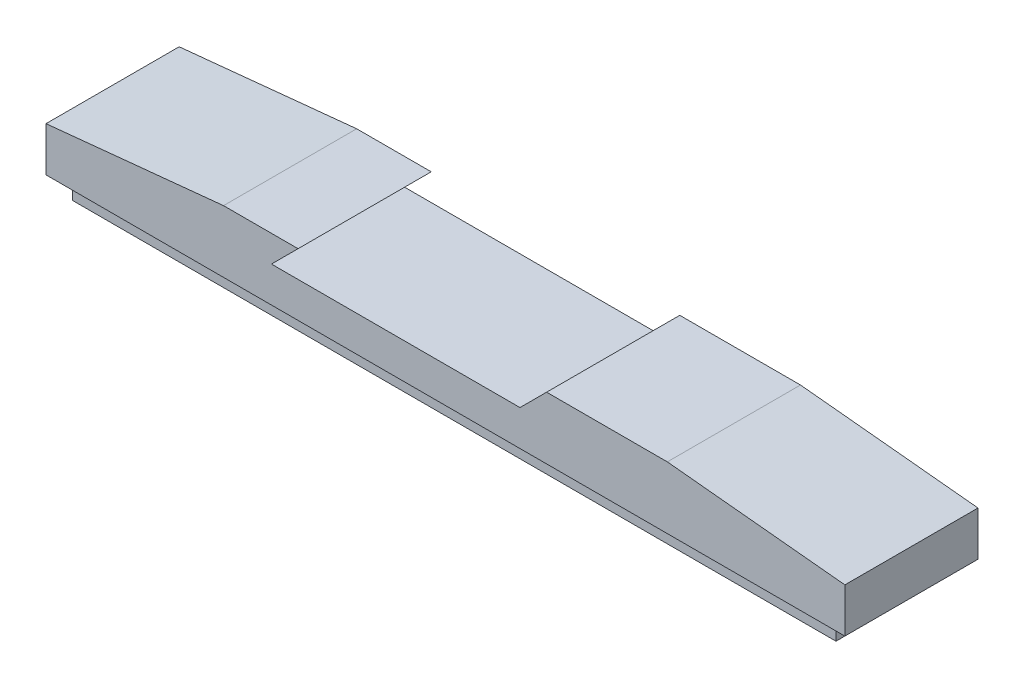
ISO-10303-21;
HEADER;
FILE_DESCRIPTION(('STEP AP214'),'2;1');
FILE_NAME('part.step','',(''),(''),'','','');
FILE_SCHEMA(('AUTOMOTIVE_DESIGN { 1 0 10303 214 1 1 1 1 }'));
ENDSEC;
DATA;
#1=APPLICATION_CONTEXT('core data for automotive mechanical design processes');
#2=APPLICATION_PROTOCOL_DEFINITION('international standard','automotive_design',2000,#1);
#3=PRODUCT_CONTEXT('',#1,'mechanical');
#4=PRODUCT('Part','Part','',(#3));
#5=PRODUCT_RELATED_PRODUCT_CATEGORY('part','',(#4));
#6=PRODUCT_DEFINITION_FORMATION('','',#4);
#7=PRODUCT_DEFINITION_CONTEXT('part definition',#1,'design');
#8=PRODUCT_DEFINITION('design','',#6,#7);
#9=PRODUCT_DEFINITION_SHAPE('','',#8);
#10=(LENGTH_UNIT() NAMED_UNIT(*) SI_UNIT(.MILLI.,.METRE.));
#11=(NAMED_UNIT(*) PLANE_ANGLE_UNIT() SI_UNIT($,.RADIAN.));
#12=(NAMED_UNIT(*) SI_UNIT($,.STERADIAN.) SOLID_ANGLE_UNIT());
#13=UNCERTAINTY_MEASURE_WITH_UNIT(LENGTH_MEASURE(1.E-05),#10,'distance_accuracy_value','');
#14=(GEOMETRIC_REPRESENTATION_CONTEXT(3) GLOBAL_UNCERTAINTY_ASSIGNED_CONTEXT((#13)) GLOBAL_UNIT_ASSIGNED_CONTEXT((#10,
#11,#12)) REPRESENTATION_CONTEXT('',''));
#15=CARTESIAN_POINT('',(0.,0.,0.));
#16=DIRECTION('',(0.,0.,1.));
#17=DIRECTION('',(1.,0.,0.));
#18=AXIS2_PLACEMENT_3D('',#15,#16,#17);
#19=CARTESIAN_POINT('',(0.,0.,37.5));
#20=DIRECTION('',(0.,1.,0.));
#21=DIRECTION('',(0.,0.,1.));
#22=AXIS2_PLACEMENT_3D('',#19,#20,#21);
#23=PLANE('',#22);
#24=DIRECTION('',(1.,0.,0.));
#25=VECTOR('',#24,1.);
#26=CARTESIAN_POINT('',(0.,0.,-12.5));
#27=LINE('',#26,#25);
#28=CARTESIAN_POINT('',(0.,0.,-12.5));
#29=VERTEX_POINT('',#28);
#30=CARTESIAN_POINT('',(430.,0.,-12.5));
#31=VERTEX_POINT('',#30);
#32=EDGE_CURVE('E57',#29,#31,#27,.T.);
#33=ORIENTED_EDGE('',*,*,#32,.F.);
#34=DIRECTION('',(0.,0.,-1.));
#35=VECTOR('',#34,1.);
#36=CARTESIAN_POINT('',(0.,0.,37.5));
#37=LINE('',#36,#35);
#38=CARTESIAN_POINT('',(0.,0.,-37.5));
#39=VERTEX_POINT('',#38);
#40=EDGE_CURVE('E156',#29,#39,#37,.T.);
#41=ORIENTED_EDGE('',*,*,#40,.T.);
#42=DIRECTION('',(1.,0.,0.));
#43=VECTOR('',#42,1.);
#44=CARTESIAN_POINT('',(0.,0.,-37.5));
#45=LINE('',#44,#43);
#46=CARTESIAN_POINT('',(450.,0.,-37.5));
#47=VERTEX_POINT('',#46);
#48=EDGE_CURVE('E190',#39,#47,#45,.T.);
#49=ORIENTED_EDGE('',*,*,#48,.T.);
#50=DIRECTION('',(0.,0.,-1.));
#51=VECTOR('',#50,1.);
#52=CARTESIAN_POINT('',(450.,0.,37.5));
#53=LINE('',#52,#51);
#54=CARTESIAN_POINT('',(450.,0.,37.5));
#55=VERTEX_POINT('',#54);
#56=EDGE_CURVE('E157',#55,#47,#53,.T.);
#57=ORIENTED_EDGE('',*,*,#56,.F.);
#58=DIRECTION('',(1.,0.,0.));
#59=VECTOR('',#58,1.);
#60=CARTESIAN_POINT('',(0.,0.,37.5));
#61=LINE('',#60,#59);
#62=CARTESIAN_POINT('',(0.,0.,37.5));
#63=VERTEX_POINT('',#62);
#64=EDGE_CURVE('E138',#63,#55,#61,.T.);
#65=ORIENTED_EDGE('',*,*,#64,.F.);
#66=CARTESIAN_POINT('',(0.,0.,12.5));
#67=VERTEX_POINT('',#66);
#68=EDGE_CURVE('E144',#63,#67,#37,.T.);
#69=ORIENTED_EDGE('',*,*,#68,.T.);
#70=DIRECTION('',(1.,0.,0.));
#71=VECTOR('',#70,1.);
#72=CARTESIAN_POINT('',(0.,0.,12.5));
#73=LINE('',#72,#71);
#74=CARTESIAN_POINT('',(430.,0.,12.5));
#75=VERTEX_POINT('',#74);
#76=EDGE_CURVE('E289',#67,#75,#73,.T.);
#77=ORIENTED_EDGE('',*,*,#76,.T.);
#78=DIRECTION('',(0.,0.,-1.));
#79=VECTOR('',#78,1.);
#80=CARTESIAN_POINT('',(430.,0.,12.5));
#81=LINE('',#80,#79);
#82=EDGE_CURVE('E169',#75,#31,#81,.T.);
#83=ORIENTED_EDGE('',*,*,#82,.T.);
#84=EDGE_LOOP('',(#33,#41,#49,#57,#65,#69,#77,#83));
#85=FACE_BOUND('',#84,.T.);
#86=ADVANCED_FACE('F41',(#85),#23,.F.);
#87=CARTESIAN_POINT('',(6.93069306930693,69.3069306930693,37.5));
#88=DIRECTION('',(0.0995037190209989,0.995037190209989,0.));
#89=DIRECTION('',(-0.995037190209989,0.0995037190209989,0.));
#90=AXIS2_PLACEMENT_3D('',#87,#88,#89);
#91=PLANE('',#90);
#92=DIRECTION('',(0.995037190209989,-0.0995037190209989,0.));
#93=VECTOR('',#92,1.);
#94=CARTESIAN_POINT('',(6.93069306930693,69.3069306930693,-37.5));
#95=LINE('',#94,#93);
#96=CARTESIAN_POINT('',(350.,35.,-37.5));
#97=VERTEX_POINT('',#96);
#98=CARTESIAN_POINT('',(450.,25.,-37.5));
#99=VERTEX_POINT('',#98);
#100=EDGE_CURVE('E164',#97,#99,#95,.T.);
#101=ORIENTED_EDGE('',*,*,#100,.F.);
#102=DIRECTION('',(0.,0.,-1.));
#103=VECTOR('',#102,1.);
#104=CARTESIAN_POINT('',(350.,35.,37.5));
#105=LINE('',#104,#103);
#106=CARTESIAN_POINT('',(350.,35.,37.5));
#107=VERTEX_POINT('',#106);
#108=EDGE_CURVE('E11',#107,#97,#105,.T.);
#109=ORIENTED_EDGE('',*,*,#108,.F.);
#110=DIRECTION('',(0.995037190209989,-0.0995037190209989,0.));
#111=VECTOR('',#110,1.);
#112=CARTESIAN_POINT('',(6.93069306930693,69.3069306930693,37.5));
#113=LINE('',#112,#111);
#114=CARTESIAN_POINT('',(450.,25.,37.5));
#115=VERTEX_POINT('',#114);
#116=EDGE_CURVE('E191',#107,#115,#113,.T.);
#117=ORIENTED_EDGE('',*,*,#116,.T.);
#118=DIRECTION('',(0.,0.,-1.));
#119=VECTOR('',#118,1.);
#120=CARTESIAN_POINT('',(450.,25.,37.5));
#121=LINE('',#120,#119);
#122=EDGE_CURVE('E63',#115,#99,#121,.T.);
#123=ORIENTED_EDGE('',*,*,#122,.T.);
#124=EDGE_LOOP('',(#101,#109,#117,#123));
#125=FACE_BOUND('',#124,.T.);
#126=ADVANCED_FACE('F43',(#125),#91,.T.);
#127=CARTESIAN_POINT('',(0.,35.,37.5));
#128=DIRECTION('',(0.,1.,0.));
#129=DIRECTION('',(0.,0.,1.));
#130=AXIS2_PLACEMENT_3D('',#127,#128,#129);
#131=PLANE('',#130);
#132=DIRECTION('',(1.,0.,0.));
#133=VECTOR('',#132,1.);
#134=CARTESIAN_POINT('',(0.,35.,-37.5));
#135=LINE('',#134,#133);
#136=CARTESIAN_POINT('',(282.,35.,-37.5));
#137=VERTEX_POINT('',#136);
#138=EDGE_CURVE('E170',#137,#97,#135,.T.);
#139=ORIENTED_EDGE('',*,*,#138,.F.);
#140=DIRECTION('',(0.,0.,-1.));
#141=VECTOR('',#140,1.);
#142=CARTESIAN_POINT('',(282.,35.,37.5));
#143=LINE('',#142,#141);
#144=CARTESIAN_POINT('',(282.,35.,37.5));
#145=VERTEX_POINT('',#144);
#146=EDGE_CURVE('E47',#145,#137,#143,.T.);
#147=ORIENTED_EDGE('',*,*,#146,.F.);
#148=DIRECTION('',(1.,0.,0.));
#149=VECTOR('',#148,1.);
#150=CARTESIAN_POINT('',(0.,35.,37.5));
#151=LINE('',#150,#149);
#152=EDGE_CURVE('E227',#145,#107,#151,.T.);
#153=ORIENTED_EDGE('',*,*,#152,.T.);
#154=ORIENTED_EDGE('',*,*,#108,.T.);
#155=EDGE_LOOP('',(#139,#147,#153,#154));
#156=FACE_BOUND('',#155,.T.);
#157=ADVANCED_FACE('F212',(#156),#131,.T.);
#158=CARTESIAN_POINT('',(123.5,-123.5,37.5));
#159=DIRECTION('',(-0.707106781186547,0.707106781186548,0.));
#160=DIRECTION('',(-0.707106781186548,-0.707106781186547,0.));
#161=AXIS2_PLACEMENT_3D('',#158,#159,#160);
#162=PLANE('',#161);
#163=DIRECTION('',(0.707106781186548,0.707106781186547,0.));
#164=VECTOR('',#163,1.);
#165=CARTESIAN_POINT('',(123.5,-123.5,-37.5));
#166=LINE('',#165,#164);
#167=CARTESIAN_POINT('',(267.,20.,-37.5));
#168=VERTEX_POINT('',#167);
#169=EDGE_CURVE('E172',#168,#137,#166,.T.);
#170=ORIENTED_EDGE('',*,*,#169,.F.);
#171=DIRECTION('',(0.,0.,-1.));
#172=VECTOR('',#171,1.);
#173=CARTESIAN_POINT('',(267.,20.,37.5));
#174=LINE('',#173,#172);
#175=CARTESIAN_POINT('',(267.,20.,37.5));
#176=VERTEX_POINT('',#175);
#177=EDGE_CURVE('E201',#176,#168,#174,.T.);
#178=ORIENTED_EDGE('',*,*,#177,.F.);
#179=DIRECTION('',(0.707106781186548,0.707106781186547,0.));
#180=VECTOR('',#179,1.);
#181=CARTESIAN_POINT('',(123.5,-123.5,37.5));
#182=LINE('',#181,#180);
#183=EDGE_CURVE('E209',#176,#145,#182,.T.);
#184=ORIENTED_EDGE('',*,*,#183,.T.);
#185=ORIENTED_EDGE('',*,*,#146,.T.);
#186=EDGE_LOOP('',(#170,#178,#184,#185));
#187=FACE_BOUND('',#186,.T.);
#188=ADVANCED_FACE('F208',(#187),#162,.T.);
#189=CARTESIAN_POINT('',(0.,20.,37.5));
#190=DIRECTION('',(0.,1.,0.));
#191=DIRECTION('',(0.,0.,1.));
#192=AXIS2_PLACEMENT_3D('',#189,#190,#191);
#193=PLANE('',#192);
#194=DIRECTION('',(1.,0.,0.));
#195=VECTOR('',#194,1.);
#196=CARTESIAN_POINT('',(0.,20.,-37.5));
#197=LINE('',#196,#195);
#198=CARTESIAN_POINT('',(127.,20.,-37.5));
#199=VERTEX_POINT('',#198);
#200=EDGE_CURVE('E171',#199,#168,#197,.T.);
#201=ORIENTED_EDGE('',*,*,#200,.F.);
#202=DIRECTION('',(0.,0.,-1.));
#203=VECTOR('',#202,1.);
#204=CARTESIAN_POINT('',(127.,20.,37.5));
#205=LINE('',#204,#203);
#206=CARTESIAN_POINT('',(127.,20.,37.5));
#207=VERTEX_POINT('',#206);
#208=EDGE_CURVE('E203',#207,#199,#205,.T.);
#209=ORIENTED_EDGE('',*,*,#208,.F.);
#210=DIRECTION('',(1.,0.,0.));
#211=VECTOR('',#210,1.);
#212=CARTESIAN_POINT('',(0.,20.,37.5));
#213=LINE('',#212,#211);
#214=EDGE_CURVE('E224',#207,#176,#213,.T.);
#215=ORIENTED_EDGE('',*,*,#214,.T.);
#216=ORIENTED_EDGE('',*,*,#177,.T.);
#217=EDGE_LOOP('',(#201,#209,#215,#216));
#218=FACE_BOUND('',#217,.T.);
#219=ADVANCED_FACE('F219',(#218),#193,.T.);
#220=CARTESIAN_POINT('',(53.4999999999999,-53.5,37.5));
#221=DIRECTION('',(0.707106781186547,-0.707106781186548,0.));
#222=DIRECTION('',(0.707106781186548,0.707106781186547,0.));
#223=AXIS2_PLACEMENT_3D('',#220,#221,#222);
#224=PLANE('',#223);
#225=DIRECTION('',(-0.707106781186548,-0.707106781186547,0.));
#226=VECTOR('',#225,1.);
#227=CARTESIAN_POINT('',(53.4999999999999,-53.5,-37.5));
#228=LINE('',#227,#226);
#229=CARTESIAN_POINT('',(142.,35.,-37.5));
#230=VERTEX_POINT('',#229);
#231=EDGE_CURVE('E180',#230,#199,#228,.T.);
#232=ORIENTED_EDGE('',*,*,#231,.F.);
#233=DIRECTION('',(0.,0.,-1.));
#234=VECTOR('',#233,1.);
#235=CARTESIAN_POINT('',(142.,35.,37.5));
#236=LINE('',#235,#234);
#237=CARTESIAN_POINT('',(142.,35.,37.5));
#238=VERTEX_POINT('',#237);
#239=EDGE_CURVE('E200',#238,#230,#236,.T.);
#240=ORIENTED_EDGE('',*,*,#239,.F.);
#241=DIRECTION('',(-0.707106781186548,-0.707106781186547,0.));
#242=VECTOR('',#241,1.);
#243=CARTESIAN_POINT('',(53.4999999999999,-53.5,37.5));
#244=LINE('',#243,#242);
#245=EDGE_CURVE('E230',#238,#207,#244,.T.);
#246=ORIENTED_EDGE('',*,*,#245,.T.);
#247=ORIENTED_EDGE('',*,*,#208,.T.);
#248=EDGE_LOOP('',(#232,#240,#246,#247));
#249=FACE_BOUND('',#248,.T.);
#250=ADVANCED_FACE('F325',(#249),#224,.T.);
#251=CARTESIAN_POINT('',(0.,35.,37.5));
#252=DIRECTION('',(0.,1.,0.));
#253=DIRECTION('',(0.,0.,1.));
#254=AXIS2_PLACEMENT_3D('',#251,#252,#253);
#255=PLANE('',#254);
#256=DIRECTION('',(1.,0.,0.));
#257=VECTOR('',#256,1.);
#258=CARTESIAN_POINT('',(0.,35.,-37.5));
#259=LINE('',#258,#257);
#260=CARTESIAN_POINT('',(100.,35.,-37.5));
#261=VERTEX_POINT('',#260);
#262=EDGE_CURVE('E179',#261,#230,#259,.T.);
#263=ORIENTED_EDGE('',*,*,#262,.F.);
#264=DIRECTION('',(0.,0.,-1.));
#265=VECTOR('',#264,1.);
#266=CARTESIAN_POINT('',(100.,35.,37.5));
#267=LINE('',#266,#265);
#268=CARTESIAN_POINT('',(100.,35.,37.5));
#269=VERTEX_POINT('',#268);
#270=EDGE_CURVE('E197',#269,#261,#267,.T.);
#271=ORIENTED_EDGE('',*,*,#270,.F.);
#272=DIRECTION('',(1.,0.,0.));
#273=VECTOR('',#272,1.);
#274=CARTESIAN_POINT('',(0.,35.,37.5));
#275=LINE('',#274,#273);
#276=EDGE_CURVE('E232',#269,#238,#275,.T.);
#277=ORIENTED_EDGE('',*,*,#276,.T.);
#278=ORIENTED_EDGE('',*,*,#239,.T.);
#279=EDGE_LOOP('',(#263,#271,#277,#278));
#280=FACE_BOUND('',#279,.T.);
#281=ADVANCED_FACE('F317',(#280),#255,.T.);
#282=CARTESIAN_POINT('',(-2.47524752475248,24.7524752475248,37.5));
#283=DIRECTION('',(-0.0995037190209989,0.995037190209989,0.));
#284=DIRECTION('',(-0.995037190209989,-0.099503719020999,0.));
#285=AXIS2_PLACEMENT_3D('',#282,#283,#284);
#286=PLANE('',#285);
#287=DIRECTION('',(0.995037190209989,0.099503719020999,0.));
#288=VECTOR('',#287,1.);
#289=CARTESIAN_POINT('',(-2.47524752475248,24.7524752475248,-37.5));
#290=LINE('',#289,#288);
#291=CARTESIAN_POINT('',(0.,25.,-37.5));
#292=VERTEX_POINT('',#291);
#293=EDGE_CURVE('E181',#292,#261,#290,.T.);
#294=ORIENTED_EDGE('',*,*,#293,.F.);
#295=DIRECTION('',(0.,0.,-1.));
#296=VECTOR('',#295,1.);
#297=CARTESIAN_POINT('',(0.,25.,37.5));
#298=LINE('',#297,#296);
#299=CARTESIAN_POINT('',(0.,25.,37.5));
#300=VERTEX_POINT('',#299);
#301=EDGE_CURVE('E154',#300,#292,#298,.T.);
#302=ORIENTED_EDGE('',*,*,#301,.F.);
#303=DIRECTION('',(0.995037190209989,0.099503719020999,0.));
#304=VECTOR('',#303,1.);
#305=CARTESIAN_POINT('',(-2.47524752475248,24.7524752475248,37.5));
#306=LINE('',#305,#304);
#307=EDGE_CURVE('E139',#300,#269,#306,.T.);
#308=ORIENTED_EDGE('',*,*,#307,.T.);
#309=ORIENTED_EDGE('',*,*,#270,.T.);
#310=EDGE_LOOP('',(#294,#302,#308,#309));
#311=FACE_BOUND('',#310,.T.);
#312=ADVANCED_FACE('F236',(#311),#286,.T.);
#313=CARTESIAN_POINT('',(0.,0.,37.5));
#314=DIRECTION('',(1.,0.,0.));
#315=DIRECTION('',(0.,1.,0.));
#316=AXIS2_PLACEMENT_3D('',#313,#314,#315);
#317=PLANE('',#316);
#318=DIRECTION('',(0.,-1.,0.));
#319=VECTOR('',#318,1.);
#320=CARTESIAN_POINT('',(0.,0.,-37.5));
#321=LINE('',#320,#319);
#322=EDGE_CURVE('E187',#292,#39,#321,.T.);
#323=ORIENTED_EDGE('',*,*,#322,.T.);
#324=ORIENTED_EDGE('',*,*,#40,.F.);
#325=DIRECTION('',(0.,-1.,0.));
#326=VECTOR('',#325,1.);
#327=CARTESIAN_POINT('',(0.,0.,-12.5));
#328=LINE('',#327,#326);
#329=CARTESIAN_POINT('',(0.,-10.,-12.5));
#330=VERTEX_POINT('',#329);
#331=EDGE_CURVE('E250',#29,#330,#328,.T.);
#332=ORIENTED_EDGE('',*,*,#331,.T.);
#333=DIRECTION('',(0.,0.,-1.));
#334=VECTOR('',#333,1.);
#335=CARTESIAN_POINT('',(0.,-10.,22.5));
#336=LINE('',#335,#334);
#337=CARTESIAN_POINT('',(0.,-10.,-22.5));
#338=VERTEX_POINT('',#337);
#339=EDGE_CURVE('E498',#330,#338,#336,.T.);
#340=ORIENTED_EDGE('',*,*,#339,.T.);
#341=DIRECTION('',(0.,-1.,0.));
#342=VECTOR('',#341,1.);
#343=CARTESIAN_POINT('',(0.,0.,-22.5));
#344=LINE('',#343,#342);
#345=CARTESIAN_POINT('',(0.,-20.,-22.5));
#346=VERTEX_POINT('',#345);
#347=EDGE_CURVE('E486',#338,#346,#344,.T.);
#348=ORIENTED_EDGE('',*,*,#347,.T.);
#349=DIRECTION('',(0.,0.,-1.));
#350=VECTOR('',#349,1.);
#351=CARTESIAN_POINT('',(0.,-20.,22.5));
#352=LINE('',#351,#350);
#353=CARTESIAN_POINT('',(0.,-20.,22.5));
#354=VERTEX_POINT('',#353);
#355=EDGE_CURVE('E499',#354,#346,#352,.T.);
#356=ORIENTED_EDGE('',*,*,#355,.F.);
#357=DIRECTION('',(0.,-1.,0.));
#358=VECTOR('',#357,1.);
#359=CARTESIAN_POINT('',(0.,0.,22.5));
#360=LINE('',#359,#358);
#361=CARTESIAN_POINT('',(0.,-10.,22.5));
#362=VERTEX_POINT('',#361);
#363=EDGE_CURVE('E519',#362,#354,#360,.T.);
#364=ORIENTED_EDGE('',*,*,#363,.F.);
#365=CARTESIAN_POINT('',(0.,-10.,12.5));
#366=VERTEX_POINT('',#365);
#367=EDGE_CURVE('E502',#362,#366,#336,.T.);
#368=ORIENTED_EDGE('',*,*,#367,.T.);
#369=DIRECTION('',(0.,-1.,0.));
#370=VECTOR('',#369,1.);
#371=CARTESIAN_POINT('',(0.,0.,12.5));
#372=LINE('',#371,#370);
#373=EDGE_CURVE('E151',#67,#366,#372,.T.);
#374=ORIENTED_EDGE('',*,*,#373,.F.);
#375=ORIENTED_EDGE('',*,*,#68,.F.);
#376=DIRECTION('',(0.,-1.,0.));
#377=VECTOR('',#376,1.);
#378=CARTESIAN_POINT('',(0.,0.,37.5));
#379=LINE('',#378,#377);
#380=EDGE_CURVE('E132',#300,#63,#379,.T.);
#381=ORIENTED_EDGE('',*,*,#380,.F.);
#382=ORIENTED_EDGE('',*,*,#301,.T.);
#383=EDGE_LOOP('',(#323,#324,#332,#340,#348,#356,#364,#368,#374,#375,#381,#382));
#384=FACE_BOUND('',#383,.T.);
#385=ADVANCED_FACE('F150',(#384),#317,.F.);
#386=CARTESIAN_POINT('',(450.,0.,37.5));
#387=DIRECTION('',(1.,0.,0.));
#388=DIRECTION('',(0.,0.,-1.));
#389=AXIS2_PLACEMENT_3D('',#386,#387,#388);
#390=PLANE('',#389);
#391=DIRECTION('',(0.,-1.,0.));
#392=VECTOR('',#391,1.);
#393=CARTESIAN_POINT('',(450.,0.,-37.5));
#394=LINE('',#393,#392);
#395=EDGE_CURVE('E188',#99,#47,#394,.T.);
#396=ORIENTED_EDGE('',*,*,#395,.F.);
#397=ORIENTED_EDGE('',*,*,#122,.F.);
#398=DIRECTION('',(0.,-1.,0.));
#399=VECTOR('',#398,1.);
#400=CARTESIAN_POINT('',(450.,0.,37.5));
#401=LINE('',#400,#399);
#402=EDGE_CURVE('E159',#115,#55,#401,.T.);
#403=ORIENTED_EDGE('',*,*,#402,.T.);
#404=ORIENTED_EDGE('',*,*,#56,.T.);
#405=EDGE_LOOP('',(#396,#397,#403,#404));
#406=FACE_BOUND('',#405,.T.);
#407=ADVANCED_FACE('F298',(#406),#390,.T.);
#408=CARTESIAN_POINT('',(0.,0.,37.5));
#409=DIRECTION('',(0.,0.,1.));
#410=DIRECTION('',(1.,0.,0.));
#411=AXIS2_PLACEMENT_3D('',#408,#409,#410);
#412=PLANE('',#411);
#413=ORIENTED_EDGE('',*,*,#116,.F.);
#414=ORIENTED_EDGE('',*,*,#152,.F.);
#415=ORIENTED_EDGE('',*,*,#183,.F.);
#416=ORIENTED_EDGE('',*,*,#214,.F.);
#417=ORIENTED_EDGE('',*,*,#245,.F.);
#418=ORIENTED_EDGE('',*,*,#276,.F.);
#419=ORIENTED_EDGE('',*,*,#307,.F.);
#420=ORIENTED_EDGE('',*,*,#380,.T.);
#421=ORIENTED_EDGE('',*,*,#64,.T.);
#422=ORIENTED_EDGE('',*,*,#402,.F.);
#423=EDGE_LOOP('',(#413,#414,#415,#416,#417,#418,#419,#420,#421,#422));
#424=FACE_BOUND('',#423,.T.);
#425=ADVANCED_FACE('F135',(#424),#412,.T.);
#426=CARTESIAN_POINT('',(0.,0.,-37.5));
#427=DIRECTION('',(0.,0.,1.));
#428=DIRECTION('',(1.,0.,0.));
#429=AXIS2_PLACEMENT_3D('',#426,#427,#428);
#430=PLANE('',#429);
#431=ORIENTED_EDGE('',*,*,#100,.T.);
#432=ORIENTED_EDGE('',*,*,#395,.T.);
#433=ORIENTED_EDGE('',*,*,#48,.F.);
#434=ORIENTED_EDGE('',*,*,#322,.F.);
#435=ORIENTED_EDGE('',*,*,#293,.T.);
#436=ORIENTED_EDGE('',*,*,#262,.T.);
#437=ORIENTED_EDGE('',*,*,#231,.T.);
#438=ORIENTED_EDGE('',*,*,#200,.T.);
#439=ORIENTED_EDGE('',*,*,#169,.T.);
#440=ORIENTED_EDGE('',*,*,#138,.T.);
#441=EDGE_LOOP('',(#431,#432,#433,#434,#435,#436,#437,#438,#439,#440));
#442=FACE_BOUND('',#441,.T.);
#443=ADVANCED_FACE('F216',(#442),#430,.F.);
#444=CARTESIAN_POINT('',(430.,0.,12.5));
#445=DIRECTION('',(1.,0.,0.));
#446=DIRECTION('',(0.,0.,-1.));
#447=AXIS2_PLACEMENT_3D('',#444,#445,#446);
#448=PLANE('',#447);
#449=DIRECTION('',(0.,-1.,0.));
#450=VECTOR('',#449,1.);
#451=CARTESIAN_POINT('',(430.,0.,-12.5));
#452=LINE('',#451,#450);
#453=CARTESIAN_POINT('',(430.,-10.,-12.5));
#454=VERTEX_POINT('',#453);
#455=EDGE_CURVE('E282',#31,#454,#452,.T.);
#456=ORIENTED_EDGE('',*,*,#455,.F.);
#457=ORIENTED_EDGE('',*,*,#82,.F.);
#458=DIRECTION('',(0.,-1.,0.));
#459=VECTOR('',#458,1.);
#460=CARTESIAN_POINT('',(430.,0.,12.5));
#461=LINE('',#460,#459);
#462=CARTESIAN_POINT('',(430.,-10.,12.5));
#463=VERTEX_POINT('',#462);
#464=EDGE_CURVE('E290',#75,#463,#461,.T.);
#465=ORIENTED_EDGE('',*,*,#464,.T.);
#466=DIRECTION('',(0.,0.,-1.));
#467=VECTOR('',#466,1.);
#468=CARTESIAN_POINT('',(430.,-10.,22.5));
#469=LINE('',#468,#467);
#470=CARTESIAN_POINT('',(430.,-10.,22.5));
#471=VERTEX_POINT('',#470);
#472=EDGE_CURVE('E267',#471,#463,#469,.T.);
#473=ORIENTED_EDGE('',*,*,#472,.F.);
#474=DIRECTION('',(0.,-1.,0.));
#475=VECTOR('',#474,1.);
#476=CARTESIAN_POINT('',(430.,0.,22.5));
#477=LINE('',#476,#475);
#478=CARTESIAN_POINT('',(430.,-20.,22.5));
#479=VERTEX_POINT('',#478);
#480=EDGE_CURVE('E494',#471,#479,#477,.T.);
#481=ORIENTED_EDGE('',*,*,#480,.T.);
#482=DIRECTION('',(0.,0.,-1.));
#483=VECTOR('',#482,1.);
#484=CARTESIAN_POINT('',(430.,-20.,22.5));
#485=LINE('',#484,#483);
#486=CARTESIAN_POINT('',(430.,-20.,-22.5));
#487=VERTEX_POINT('',#486);
#488=EDGE_CURVE('E497',#479,#487,#485,.T.);
#489=ORIENTED_EDGE('',*,*,#488,.T.);
#490=DIRECTION('',(0.,-1.,0.));
#491=VECTOR('',#490,1.);
#492=CARTESIAN_POINT('',(430.,0.,-22.5));
#493=LINE('',#492,#491);
#494=CARTESIAN_POINT('',(430.,-10.,-22.5));
#495=VERTEX_POINT('',#494);
#496=EDGE_CURVE('E474',#495,#487,#493,.T.);
#497=ORIENTED_EDGE('',*,*,#496,.F.);
#498=EDGE_CURVE('E284',#454,#495,#469,.T.);
#499=ORIENTED_EDGE('',*,*,#498,.F.);
#500=EDGE_LOOP('',(#456,#457,#465,#473,#481,#489,#497,#499));
#501=FACE_BOUND('',#500,.T.);
#502=ADVANCED_FACE('F287',(#501),#448,.T.);
#503=CARTESIAN_POINT('',(0.,0.,12.5));
#504=DIRECTION('',(0.,0.,1.));
#505=DIRECTION('',(1.,0.,0.));
#506=AXIS2_PLACEMENT_3D('',#503,#504,#505);
#507=PLANE('',#506);
#508=ORIENTED_EDGE('',*,*,#464,.F.);
#509=ORIENTED_EDGE('',*,*,#76,.F.);
#510=ORIENTED_EDGE('',*,*,#373,.T.);
#511=DIRECTION('',(1.,0.,0.));
#512=VECTOR('',#511,1.);
#513=CARTESIAN_POINT('',(0.,-10.,12.5));
#514=LINE('',#513,#512);
#515=EDGE_CURVE('E272',#366,#463,#514,.T.);
#516=ORIENTED_EDGE('',*,*,#515,.T.);
#517=EDGE_LOOP('',(#508,#509,#510,#516));
#518=FACE_BOUND('',#517,.T.);
#519=ADVANCED_FACE('F288',(#518),#507,.T.);
#520=CARTESIAN_POINT('',(0.,0.,-12.5));
#521=DIRECTION('',(0.,0.,1.));
#522=DIRECTION('',(1.,0.,0.));
#523=AXIS2_PLACEMENT_3D('',#520,#521,#522);
#524=PLANE('',#523);
#525=ORIENTED_EDGE('',*,*,#455,.T.);
#526=DIRECTION('',(1.,0.,0.));
#527=VECTOR('',#526,1.);
#528=CARTESIAN_POINT('',(0.,-10.,-12.5));
#529=LINE('',#528,#527);
#530=EDGE_CURVE('E256',#330,#454,#529,.T.);
#531=ORIENTED_EDGE('',*,*,#530,.F.);
#532=ORIENTED_EDGE('',*,*,#331,.F.);
#533=ORIENTED_EDGE('',*,*,#32,.T.);
#534=EDGE_LOOP('',(#525,#531,#532,#533));
#535=FACE_BOUND('',#534,.T.);
#536=ADVANCED_FACE('F407',(#535),#524,.F.);
#537=CARTESIAN_POINT('',(0.,-10.,22.5));
#538=DIRECTION('',(0.,1.,0.));
#539=DIRECTION('',(0.,0.,1.));
#540=AXIS2_PLACEMENT_3D('',#537,#538,#539);
#541=PLANE('',#540);
#542=ORIENTED_EDGE('',*,*,#515,.F.);
#543=ORIENTED_EDGE('',*,*,#367,.F.);
#544=DIRECTION('',(1.,0.,0.));
#545=VECTOR('',#544,1.);
#546=CARTESIAN_POINT('',(0.,-10.,22.5));
#547=LINE('',#546,#545);
#548=EDGE_CURVE('E277',#362,#471,#547,.T.);
#549=ORIENTED_EDGE('',*,*,#548,.T.);
#550=ORIENTED_EDGE('',*,*,#472,.T.);
#551=EDGE_LOOP('',(#542,#543,#549,#550));
#552=FACE_BOUND('',#551,.T.);
#553=ADVANCED_FACE('F271',(#552),#541,.T.);
#554=ORIENTED_EDGE('',*,*,#339,.F.);
#555=ORIENTED_EDGE('',*,*,#530,.T.);
#556=ORIENTED_EDGE('',*,*,#498,.T.);
#557=DIRECTION('',(1.,0.,0.));
#558=VECTOR('',#557,1.);
#559=CARTESIAN_POINT('',(0.,-10.,-22.5));
#560=LINE('',#559,#558);
#561=EDGE_CURVE('E485',#338,#495,#560,.T.);
#562=ORIENTED_EDGE('',*,*,#561,.F.);
#563=EDGE_LOOP('',(#554,#555,#556,#562));
#564=FACE_BOUND('',#563,.T.);
#565=ADVANCED_FACE('F423',(#564),#541,.T.);
#566=CARTESIAN_POINT('',(0.,-20.,22.5));
#567=DIRECTION('',(0.,1.,0.));
#568=DIRECTION('',(0.,0.,1.));
#569=AXIS2_PLACEMENT_3D('',#566,#567,#568);
#570=PLANE('',#569);
#571=DIRECTION('',(1.,0.,0.));
#572=VECTOR('',#571,1.);
#573=CARTESIAN_POINT('',(0.,-20.,-22.5));
#574=LINE('',#573,#572);
#575=EDGE_CURVE('E479',#346,#487,#574,.T.);
#576=ORIENTED_EDGE('',*,*,#575,.T.);
#577=ORIENTED_EDGE('',*,*,#488,.F.);
#578=DIRECTION('',(1.,0.,0.));
#579=VECTOR('',#578,1.);
#580=CARTESIAN_POINT('',(0.,-20.,22.5));
#581=LINE('',#580,#579);
#582=EDGE_CURVE('E487',#354,#479,#581,.T.);
#583=ORIENTED_EDGE('',*,*,#582,.F.);
#584=ORIENTED_EDGE('',*,*,#355,.T.);
#585=EDGE_LOOP('',(#576,#577,#583,#584));
#586=FACE_BOUND('',#585,.T.);
#587=ADVANCED_FACE('F427',(#586),#570,.F.);
#588=CARTESIAN_POINT('',(0.,0.,22.5));
#589=DIRECTION('',(0.,0.,1.));
#590=DIRECTION('',(1.,0.,0.));
#591=AXIS2_PLACEMENT_3D('',#588,#589,#590);
#592=PLANE('',#591);
#593=ORIENTED_EDGE('',*,*,#480,.F.);
#594=ORIENTED_EDGE('',*,*,#548,.F.);
#595=ORIENTED_EDGE('',*,*,#363,.T.);
#596=ORIENTED_EDGE('',*,*,#582,.T.);
#597=EDGE_LOOP('',(#593,#594,#595,#596));
#598=FACE_BOUND('',#597,.T.);
#599=ADVANCED_FACE('F436',(#598),#592,.T.);
#600=CARTESIAN_POINT('',(0.,0.,-22.5));
#601=DIRECTION('',(0.,0.,1.));
#602=DIRECTION('',(1.,0.,0.));
#603=AXIS2_PLACEMENT_3D('',#600,#601,#602);
#604=PLANE('',#603);
#605=ORIENTED_EDGE('',*,*,#496,.T.);
#606=ORIENTED_EDGE('',*,*,#575,.F.);
#607=ORIENTED_EDGE('',*,*,#347,.F.);
#608=ORIENTED_EDGE('',*,*,#561,.T.);
#609=EDGE_LOOP('',(#605,#606,#607,#608));
#610=FACE_BOUND('',#609,.T.);
#611=ADVANCED_FACE('F443',(#610),#604,.F.);
#612=CLOSED_SHELL('',(#86,#126,#157,#188,#219,#250,#281,#312,#385,#407,#425,#443,#502,#519,#536,
#553,#565,#587,#599,#611));
#613=MANIFOLD_SOLID_BREP('B2',#612);
#614=ADVANCED_BREP_SHAPE_REPRESENTATION('',(#18,#613),#14);
#615=SHAPE_DEFINITION_REPRESENTATION(#9,#614);
ENDSEC;
END-ISO-10303-21;
